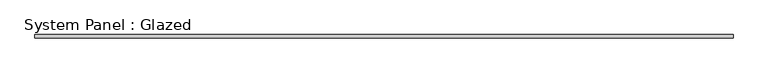
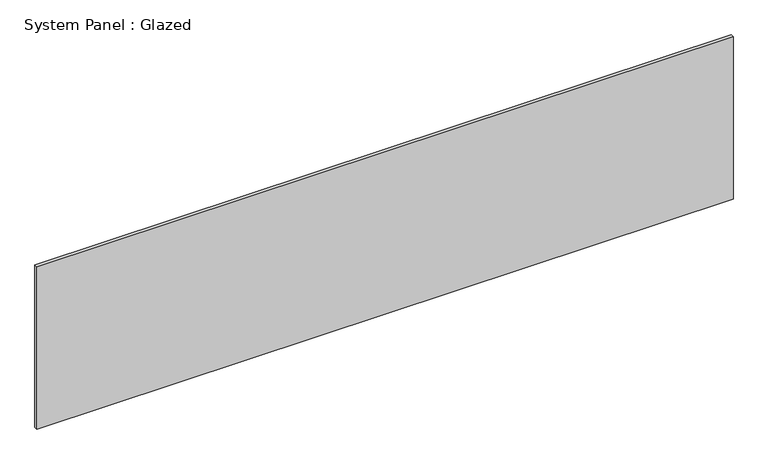
"""IFC4 building model written with IfcOpenShell, lengths in millimetres: plate geometry, System Panel : Glazed."""

from ifc_helpers import new_model, si_unit, origin, origin_with_axes, place, context, project, spatial, polyline, outline, extrude, source, transform, mapped, element, save


def system_panel_glazed_51f6397d(model_context):
    return source(origin(), model_context, "Body", "SweptSolid", [
        extrude(outline(polyline([(2476.5, 19.05), (-2476.5, 19.05), (-2476.5, 44.45), (2476.5, 44.45), (2476.5, 19.05)])), origin_with_axes(), (0.0, 0.0, 1.0), 1219.2),
    ])


if __name__ == "__main__":
    model = new_model("IFC4")
    model_context = context("Model", 3, world=origin())
    ifc_project = project(units=[si_unit("LENGTHUNIT", "METRE", prefix="MILLI")], contexts=[model_context])
    site = spatial("IfcSite", under=ifc_project)
    building = spatial("IfcBuilding", under=site)
    placement = place(None, origin())
    system_panel_glazed_shape = system_panel_glazed_51f6397d(model_context)
    element("IfcPlate", 1, ObjectType="System Panel : Glazed", at=placement, inside=building, context=model_context, shape_type="MappedRepresentation", body=[
        mapped(system_panel_glazed_shape, transform((0.0, 0.0, 0.0), x_axis=(1.0, 0.0, 0.0), y_axis=(0.0, 1.0, 0.0), z_axis=(0.0, 0.0, 1.0))),
    ])
    save(model, "model.ifc")

# Revit data of these elements
# Type "System Panel : Glazed"
#   Construction Type Id = "GSP4R"
#   Analytic Construction = "1/8 in Pilkington single glazing"
#   Visual Light Transmittance = 0.9
#   Solar Heat Gain Coefficient = 0.86
#   Heat Transfer Coefficient (U) = 1.18115 BTU/(h·ft²·°F)
# Element 1 (IfcPlate, "System Panel : Glazed")
#   Materials on its faces: "Glass"
# Materials
#   "Glass": class "Glass", colour RGB 0 128 192, transparency 0.75, Description = "Soda Lime Glass", Cost = 0
